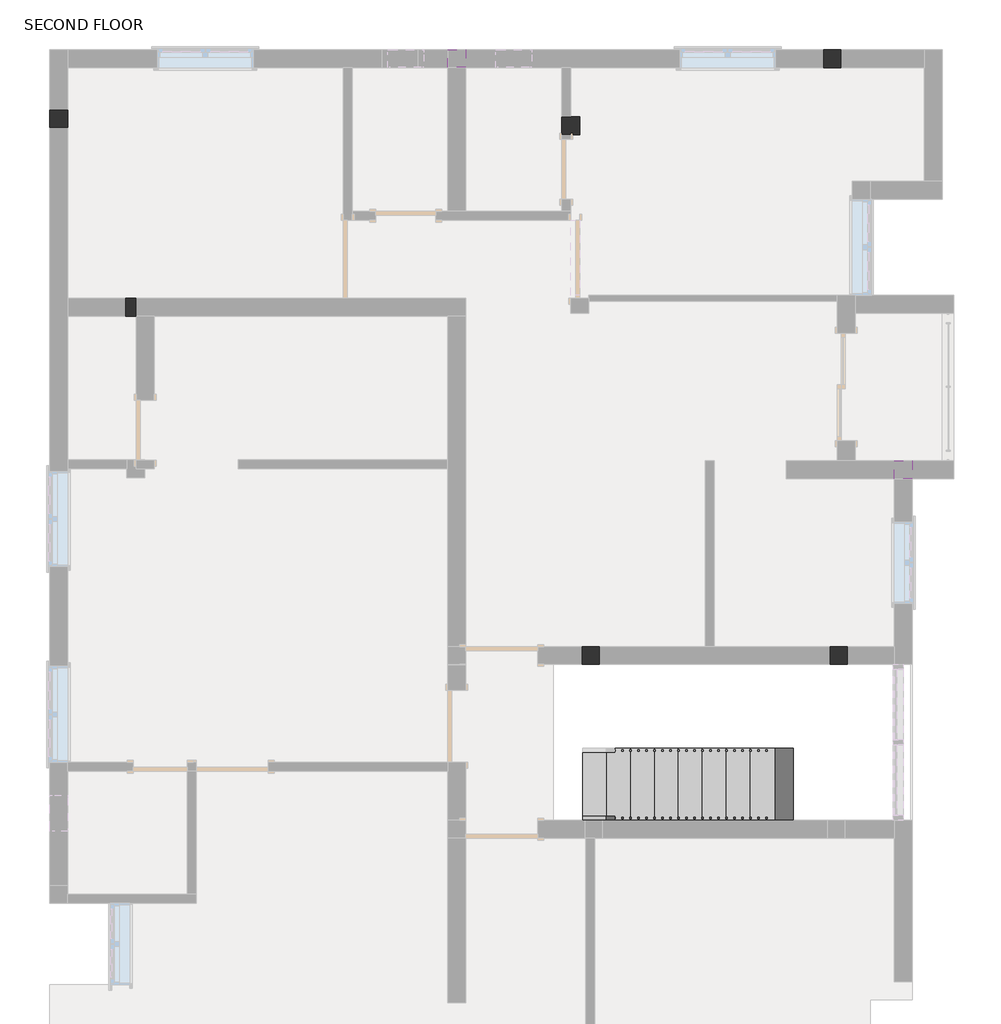
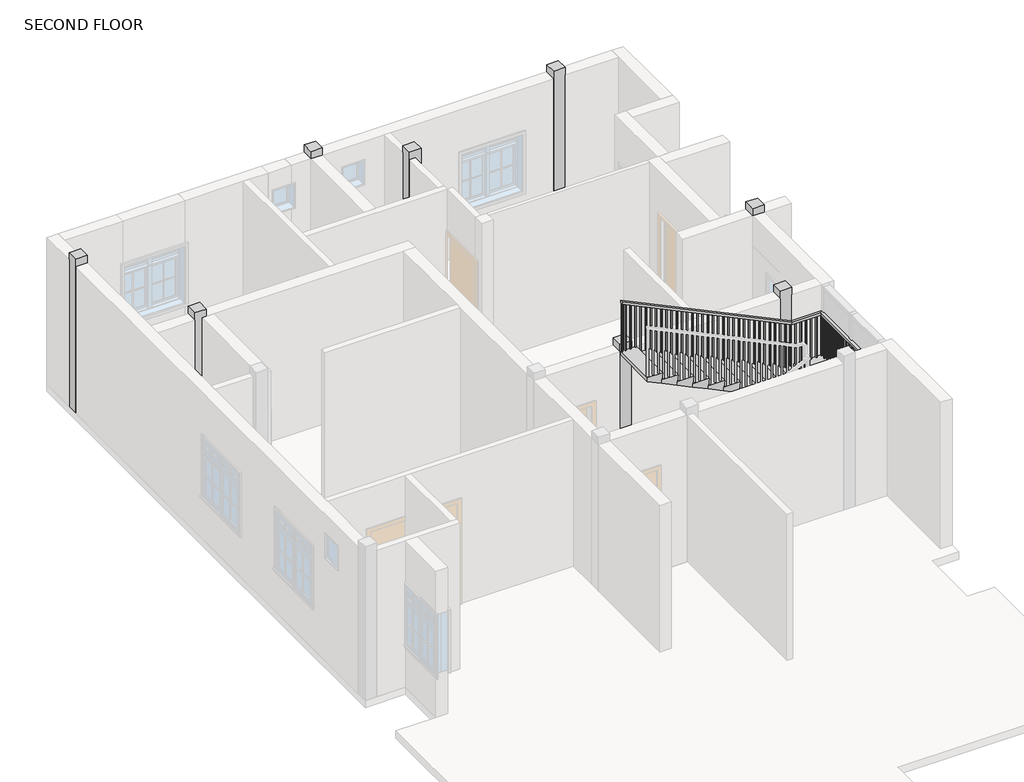
# One storey, part 4 of 6: 8 columns, 1 railing, 1 stair flight.
"""IFC4 building model written with IfcOpenShell, lengths in millimetres."""

from ifc_helpers import new_model, si_unit, frame, origin, place, context, project, spatial, polyline, outline, extrude, faceted_brep, element, save

model = new_model("IFC4")

# Units and contexts
model_context = context("Model", 3, world=origin())
ifc_project = project(units=[si_unit("LENGTHUNIT", "METRE", prefix="MILLI")], contexts=[model_context])

# Site, building, storey
site = spatial("IfcSite", under=ifc_project)
building = spatial("IfcBuilding", under=site)
storey = spatial("IfcBuildingStorey", under=building, Name="SECOND FLOOR", Elevation=6400.8)

# Columns
placement = place(None, origin())
element("IfcColumn", 1, ObjectType="Rectangular Column : 9\"X9\"", at=placement, inside=storey, context=model_context, shape_type="Brep", body=[
    faceted_brep([(-6539.8865981, 8531.2343988, 6400.8), (-6539.8865981, 8302.6343988, 6400.8), (-6768.4865981, 8302.6343988, 6400.8), (-6768.4865981, 8531.2343988, 6400.8), (-6539.8865981, 8531.2343988, 9601.2), (-6539.8865981, 8302.6343988, 9601.2), (-6539.8865981, 8302.6343988, 9448.8), (-6539.8865981, 8531.2343988, 9448.8), (-6768.4865981, 8302.6343988, 9601.2), (-6768.4865981, 8302.6343988, 9448.8), (-6768.4865981, 8531.2343988, 9601.2), (-6768.4865981, 8531.2343988, 9448.8)], [[[0, 1, 2, 3]], [[4, 5, 6, 1, 0, 7]], [[5, 8, 9, 2, 1, 6]], [[8, 10, 11, 3, 2, 9]], [[10, 4, 7, 0, 3, 11]], [[4, 10, 8, 5]]]),
])
element("IfcColumn", 2, ObjectType="Rectangular Column : 9\"X9\"", at=placement, inside=storey, context=model_context, shape_type="Brep", body=[
    faceted_brep([(229.251657, 1705.5787587, 6400.8), (229.251657, 1476.9787587, 6400.8), (0.651657, 1476.9787587, 6400.8), (0.651657, 1705.5787587, 6400.8), (229.251657, 1705.5787587, 9601.2), (229.251657, 1476.9787587, 9601.2), (229.251657, 1476.9787587, 9448.8), (229.251657, 1705.5787587, 9448.8), (0.651657, 1476.9787587, 9601.2), (0.651657, 1476.9787587, 9448.8), (0.651657, 1705.5787587, 9601.2), (0.651657, 1705.5787587, 9448.8)], [[[0, 1, 2, 3]], [[4, 5, 6, 1, 0, 7]], [[5, 8, 9, 2, 1, 6]], [[8, 10, 11, 3, 2, 9]], [[10, 4, 7, 0, 3, 11]], [[4, 10, 8, 5]]]),
])
element("IfcColumn", 3, ObjectType="Rectangular Column : 9\"X9\"", at=placement, inside=storey, context=model_context, shape_type="Brep", body=[
    faceted_brep([(3385.1070369, 1705.5787587, 6400.8), (3385.1070369, 1476.9787587, 6400.8), (3156.5070369, 1476.9787587, 6400.8), (3156.5070369, 1705.5787587, 6400.8), (3385.1070369, 1705.5787587, 9601.2), (3385.1070369, 1476.9787587, 9601.2), (3385.1070369, 1476.9787587, 9448.8), (3385.1070369, 1705.5787587, 9448.8), (3156.5070369, 1476.9787587, 9601.2), (3156.5070369, 1476.9787587, 9448.8), (3156.5070369, 1705.5787587, 9601.2), (3156.5070369, 1705.5787587, 9448.8)], [[[0, 1, 2, 3]], [[4, 5, 6, 1, 0, 7]], [[5, 8, 9, 2, 1, 6]], [[8, 10, 11, 3, 2, 9]], [[10, 4, 7, 0, 3, 11]], [[4, 10, 8, 5]]]),
])
element("IfcColumn", 4, ObjectType="Rectangular Column : 9\"X9\"", at=placement, inside=storey, context=model_context, shape_type="SweptSolid", body=[
    extrude(outline(polyline([(4204.3134019, 4067.7787587), (4204.3134019, 3839.1787587), (3975.7134019, 3839.1787587), (3975.7134019, 4067.7787587), (4204.3134019, 4067.7787587)])), frame((0.0, 0.0, 9448.8), z_axis=(0.0, 0.0, 1.0), x_axis=(1.0, 0.0, 0.0)), (0.0, 0.0, 1.0), 152.4),
])
element("IfcColumn", 5, ObjectType="Rectangular Column : 9\"X9\"", at=placement, inside=storey, context=model_context, shape_type="Brep", body=[
    faceted_brep([(3305.8577655, 9300.1787587, 6400.8), (3305.8577655, 9071.5787587, 6400.8), (3077.2577655, 9071.5787587, 6400.8), (3077.2577655, 9300.1787587, 6400.8), (3305.8577655, 9300.1787587, 9601.2), (3305.8577655, 9071.5787587, 9601.2), (3305.8577655, 9071.5787587, 9448.8), (3305.8577655, 9300.1787587, 9448.8), (3077.2577655, 9071.5787587, 9601.2), (3077.2577655, 9071.5787587, 9448.8), (3077.2577655, 9300.1787587, 9601.2), (3077.2577655, 9300.1787587, 9448.8)], [[[0, 1, 2, 3]], [[4, 5, 6, 1, 0, 7]], [[5, 8, 9, 2, 1, 6]], [[8, 10, 11, 3, 2, 9]], [[10, 4, 7, 0, 3, 11]], [[4, 10, 8, 5]]]),
])
element("IfcColumn", 6, ObjectType="Rectangular Column : 9\"X9\"", at=placement, inside=storey, context=model_context, shape_type="Brep", body=[
    faceted_brep([(-24.7865981, 8443.0921256, 6400.8), (-24.7865981, 8214.4921256, 6400.8), (-139.0865981, 8214.4921256, 6400.8), (-253.3865981, 8214.4921256, 6400.8), (-253.3865981, 8443.0921256, 6400.8), (-139.0865981, 8443.0921256, 6400.8), (-24.7865981, 8443.0921256, 9601.2), (-24.7865981, 8214.4921256, 9601.2), (-253.3865981, 8214.4921256, 9601.2), (-253.3865981, 8214.4921256, 9448.8), (-253.3865981, 8443.0921256, 9601.2), (-253.3865981, 8443.0921256, 9448.8)], [[[0, 1, 2, 3, 4, 5]], [[6, 7, 1, 0]], [[7, 8, 9, 3, 2, 1]], [[8, 10, 11, 4, 3, 9]], [[10, 6, 0, 5, 4, 11]], [[6, 10, 8, 7]]]),
])
element("IfcColumn", 7, ObjectType="Rectangular Column : 9\"X9\"", at=placement, inside=storey, context=model_context, shape_type="Brep", body=[
    faceted_brep([(-5807.056564, 5909.2787587, 6400.8), (-5807.056564, 6137.8787587, 6400.8), (-5663.5865981, 6137.8787587, 6400.8), (-5663.5865981, 5909.2787587, 6400.8), (-5578.456564, 6137.8787587, 9601.2), (-5578.456564, 5909.2787587, 9601.2), (-5578.456564, 5909.2787587, 9448.8), (-5578.456564, 6137.8787587, 9448.8), (-5807.056564, 5909.2787587, 9601.2), (-5807.056564, 5909.2787587, 9448.8), (-5663.5865981, 5909.2787587, 9448.8), (-5807.056564, 6137.8787587, 9601.2), (-5807.056564, 6137.8787587, 9448.8), (-5663.5865981, 6137.8787587, 9448.8)], [[[0, 1, 2, 3]], [[4, 5, 6, 7]], [[5, 8, 9, 0, 3, 10, 6]], [[1, 0, 9, 8, 11, 12]], [[1, 12, 11, 4, 7, 13, 2]], [[5, 4, 11, 8]], [[10, 13, 7, 6]], [[13, 10, 3, 2]]]),
])
element("IfcColumn", 8, ObjectType="Rectangular Column : 9\"X9\"", at=placement, inside=storey, context=model_context, shape_type="SweptSolid", body=[
    extrude(outline(polyline([(-1472.5865981, 9300.1787587), (-1472.5865981, 9071.5787587), (-1701.1865981, 9071.5787587), (-1701.1865981, 9300.1787587), (-1472.5865981, 9300.1787587)])), frame((0.0, 0.0, 9448.8), z_axis=(0.0, 0.0, 1.0), x_axis=(1.0, 0.0, 0.0)), (0.0, 0.0, 1.0), 152.4),
])

# Railing
element("IfcRailing", 9, ObjectType="Handrail - Rectangular", at=placement, inside=storey, context=model_context, shape_type="SolidModel", body=[
    faceted_brep([(13.3134019, -453.4212413, 7460.6727273), (13.3134019, -453.4212413, 7404.3834559), (13.3134019, -504.2212413, 7404.3834559), (13.3134019, -504.2212413, 7460.6727273), (3061.3134019, -453.4212413, 8915.4), (3072.8147322, -453.4212413, 8864.6), (3072.8147322, -504.2212413, 8864.6), (3061.3134019, -504.2212413, 8915.4), (3924.9134019, -453.4212413, 8915.4), (3924.9134019, -453.4212413, 8864.6), (3975.7134019, -504.2212413, 8864.6), (3975.7134019, -504.2212413, 8915.4), (3924.9134019, 1426.1787587, 8915.4), (3924.9134019, 1426.1787587, 8864.6), (3975.7134019, 1476.9787587, 8864.6), (3975.7134019, 1476.9787587, 8915.4), (3366.1134019, 1426.1787587, 8915.4), (3354.6120715, 1426.1787587, 8864.6), (3354.6120715, 1476.9787587, 8864.6), (3366.1134019, 1476.9787587, 8915.4), (13.3134019, 1426.1787587, 10515.6), (13.3134019, 1476.9787587, 10515.6), (13.3134019, 1476.9787587, 10459.3107287), (13.3134019, 1426.1787587, 10459.3107287)], [[[0, 1, 2, 3]], [[1, 0, 4, 5]], [[2, 1, 5, 6]], [[3, 2, 6, 7]], [[0, 3, 7, 4]], [[5, 4, 8, 9]], [[6, 5, 9, 10]], [[7, 6, 10, 11]], [[4, 7, 11, 8]], [[9, 8, 12, 13]], [[10, 9, 13, 14]], [[11, 10, 14, 15]], [[8, 11, 15, 12]], [[13, 12, 16, 17]], [[14, 13, 17, 18]], [[15, 14, 18, 19]], [[12, 15, 19, 16]], [[20, 21, 22, 23]], [[17, 16, 20, 23]], [[18, 17, 23, 22]], [[19, 18, 22, 21]], [[16, 19, 21, 20]]]),
    extrude(outline(polyline([(10418.3965241, 99.0384019), (10427.4885696, 79.9884019), (9455.7272727, 79.9884019), (9455.7272727, 99.0384019), (10418.3965241, 99.0384019)])), frame((0.0, 1442.0537587, 0.0), z_axis=(0.0, 1.0, 0.0), x_axis=(0.0, 0.0, 1.0)), (0.0, 0.0, 1.0), 19.05),
    extrude(outline(polyline([(10369.905615, 200.6384019), (10378.9976605, 181.5884019), (9455.7272727, 181.5884019), (9455.7272727, 200.6384019), (10369.905615, 200.6384019)])), frame((0.0, 1442.0537587, 0.0), z_axis=(0.0, 1.0, 0.0), x_axis=(0.0, 0.0, 1.0)), (0.0, 0.0, 1.0), 19.05),
    extrude(outline(polyline([(10321.4147059, 302.2384019), (10330.5067514, 283.1884019), (9455.7272727, 283.1884019), (9455.7272727, 302.2384019), (10321.4147059, 302.2384019)])), frame((0.0, 1442.0537587, 0.0), z_axis=(0.0, 1.0, 0.0), x_axis=(0.0, 0.0, 1.0)), (0.0, 0.0, 1.0), 19.05),
    extrude(outline(polyline([(10272.9237969, 403.8384019), (10282.0158423, 384.7884019), (9310.2545455, 384.7884019), (9310.2545455, 403.8384019), (10272.9237969, 403.8384019)])), frame((0.0, 1442.0537587, 0.0), z_axis=(0.0, 1.0, 0.0), x_axis=(0.0, 0.0, 1.0)), (0.0, 0.0, 1.0), 19.05),
    extrude(outline(polyline([(10224.4328878, 505.4384019), (10233.5249332, 486.3884019), (9310.2545455, 486.3884019), (9310.2545455, 505.4384019), (10224.4328878, 505.4384019)])), frame((0.0, 1442.0537587, 0.0), z_axis=(0.0, 1.0, 0.0), x_axis=(0.0, 0.0, 1.0)), (0.0, 0.0, 1.0), 19.05),
    extrude(outline(polyline([(10175.9419787, 607.0384019), (10185.0340241, 587.9884019), (9310.2545455, 587.9884019), (9310.2545455, 607.0384019), (10175.9419787, 607.0384019)])), frame((0.0, 1442.0537587, 0.0), z_axis=(0.0, 1.0, 0.0), x_axis=(0.0, 0.0, 1.0)), (0.0, 0.0, 1.0), 19.05),
    extrude(outline(polyline([(10127.4510696, 708.6384019), (10136.543115, 689.5884019), (9164.7818182, 689.5884019), (9164.7818182, 708.6384019), (10127.4510696, 708.6384019)])), frame((0.0, 1442.0537587, 0.0), z_axis=(0.0, 1.0, 0.0), x_axis=(0.0, 0.0, 1.0)), (0.0, 0.0, 1.0), 19.05),
    extrude(outline(polyline([(10078.9601605, 810.2384019), (10088.0522059, 791.1884019), (9164.7818182, 791.1884019), (9164.7818182, 810.2384019), (10078.9601605, 810.2384019)])), frame((0.0, 1442.0537587, 0.0), z_axis=(0.0, 1.0, 0.0), x_axis=(0.0, 0.0, 1.0)), (0.0, 0.0, 1.0), 19.05),
    extrude(outline(polyline([(10030.4692514, 911.8384019), (10039.5612969, 892.7884019), (9164.7818182, 892.7884019), (9164.7818182, 911.8384019), (10030.4692514, 911.8384019)])), frame((0.0, 1442.0537587, 0.0), z_axis=(0.0, 1.0, 0.0), x_axis=(0.0, 0.0, 1.0)), (0.0, 0.0, 1.0), 19.05),
    extrude(outline(polyline([(9981.9783423, 1013.4384019), (9991.0703878, 994.3884019), (9019.3090909, 994.3884019), (9019.3090909, 1013.4384019), (9981.9783423, 1013.4384019)])), frame((0.0, 1442.0537587, 0.0), z_axis=(0.0, 1.0, 0.0), x_axis=(0.0, 0.0, 1.0)), (0.0, 0.0, 1.0), 19.05),
    extrude(outline(polyline([(9933.4874332, 1115.0384019), (9942.5794787, 1095.9884019), (9019.3090909, 1095.9884019), (9019.3090909, 1115.0384019), (9933.4874332, 1115.0384019)])), frame((0.0, 1442.0537587, 0.0), z_axis=(0.0, 1.0, 0.0), x_axis=(0.0, 0.0, 1.0)), (0.0, 0.0, 1.0), 19.05),
    extrude(outline(polyline([(9884.9965241, 1216.6384019), (9894.0885696, 1197.5884019), (9019.3090909, 1197.5884019), (9019.3090909, 1216.6384019), (9884.9965241, 1216.6384019)])), frame((0.0, 1442.0537587, 0.0), z_axis=(0.0, 1.0, 0.0), x_axis=(0.0, 0.0, 1.0)), (0.0, 0.0, 1.0), 19.05),
    extrude(outline(polyline([(9836.505615, 1318.2384019), (9845.5976605, 1299.1884019), (8873.8363636, 1299.1884019), (8873.8363636, 1318.2384019), (9836.505615, 1318.2384019)])), frame((0.0, 1442.0537587, 0.0), z_axis=(0.0, 1.0, 0.0), x_axis=(0.0, 0.0, 1.0)), (0.0, 0.0, 1.0), 19.05),
    extrude(outline(polyline([(9788.0147059, 1419.8384019), (9797.1067514, 1400.7884019), (8873.8363636, 1400.7884019), (8873.8363636, 1419.8384019), (9788.0147059, 1419.8384019)])), frame((0.0, 1442.0537587, 0.0), z_axis=(0.0, 1.0, 0.0), x_axis=(0.0, 0.0, 1.0)), (0.0, 0.0, 1.0), 19.05),
    extrude(outline(polyline([(9739.5237969, 1521.4384019), (9748.6158423, 1502.3884019), (8873.8363636, 1502.3884019), (8873.8363636, 1521.4384019), (9739.5237969, 1521.4384019)])), frame((0.0, 1442.0537587, 0.0), z_axis=(0.0, 1.0, 0.0), x_axis=(0.0, 0.0, 1.0)), (0.0, 0.0, 1.0), 19.05),
    extrude(outline(polyline([(9691.0328878, 1623.0384019), (9700.1249332, 1603.9884019), (8728.3636364, 1603.9884019), (8728.3636364, 1623.0384019), (9691.0328878, 1623.0384019)])), frame((0.0, 1442.0537587, 0.0), z_axis=(0.0, 1.0, 0.0), x_axis=(0.0, 0.0, 1.0)), (0.0, 0.0, 1.0), 19.05),
    extrude(outline(polyline([(9642.5419787, 1724.6384019), (9651.6340241, 1705.5884019), (8728.3636364, 1705.5884019), (8728.3636364, 1724.6384019), (9642.5419787, 1724.6384019)])), frame((0.0, 1442.0537587, 0.0), z_axis=(0.0, 1.0, 0.0), x_axis=(0.0, 0.0, 1.0)), (0.0, 0.0, 1.0), 19.05),
    extrude(outline(polyline([(9594.0510696, 1826.2384019), (9603.143115, 1807.1884019), (8728.3636364, 1807.1884019), (8728.3636364, 1826.2384019), (9594.0510696, 1826.2384019)])), frame((0.0, 1442.0537587, 0.0), z_axis=(0.0, 1.0, 0.0), x_axis=(0.0, 0.0, 1.0)), (0.0, 0.0, 1.0), 19.05),
    extrude(outline(polyline([(9545.5601605, 1927.8384019), (9554.6522059, 1908.7884019), (8582.8909091, 1908.7884019), (8582.8909091, 1927.8384019), (9545.5601605, 1927.8384019)])), frame((0.0, 1442.0537587, 0.0), z_axis=(0.0, 1.0, 0.0), x_axis=(0.0, 0.0, 1.0)), (0.0, 0.0, 1.0), 19.05),
    extrude(outline(polyline([(9497.0692514, 2029.4384019), (9506.1612969, 2010.3884019), (8582.8909091, 2010.3884019), (8582.8909091, 2029.4384019), (9497.0692514, 2029.4384019)])), frame((0.0, 1442.0537587, 0.0), z_axis=(0.0, 1.0, 0.0), x_axis=(0.0, 0.0, 1.0)), (0.0, 0.0, 1.0), 19.05),
    extrude(outline(polyline([(9448.5783423, 2131.0384019), (9457.6703878, 2111.9884019), (8582.8909091, 2111.9884019), (8582.8909091, 2131.0384019), (9448.5783423, 2131.0384019)])), frame((0.0, 1442.0537587, 0.0), z_axis=(0.0, 1.0, 0.0), x_axis=(0.0, 0.0, 1.0)), (0.0, 0.0, 1.0), 19.05),
    extrude(outline(polyline([(9400.0874332, 2232.6384019), (9409.1794787, 2213.5884019), (8437.4181818, 2213.5884019), (8437.4181818, 2232.6384019), (9400.0874332, 2232.6384019)])), frame((0.0, 1442.0537587, 0.0), z_axis=(0.0, 1.0, 0.0), x_axis=(0.0, 0.0, 1.0)), (0.0, 0.0, 1.0), 19.05),
    extrude(outline(polyline([(9351.5965241, 2334.2384019), (9360.6885696, 2315.1884019), (8437.4181818, 2315.1884019), (8437.4181818, 2334.2384019), (9351.5965241, 2334.2384019)])), frame((0.0, 1442.0537587, 0.0), z_axis=(0.0, 1.0, 0.0), x_axis=(0.0, 0.0, 1.0)), (0.0, 0.0, 1.0), 19.05),
    extrude(outline(polyline([(9303.105615, 2435.8384019), (9312.1976605, 2416.7884019), (8437.4181818, 2416.7884019), (8437.4181818, 2435.8384019), (9303.105615, 2435.8384019)])), frame((0.0, 1442.0537587, 0.0), z_axis=(0.0, 1.0, 0.0), x_axis=(0.0, 0.0, 1.0)), (0.0, 0.0, 1.0), 19.05),
    extrude(outline(polyline([(9254.6147059, 2537.4384019), (9263.7067514, 2518.3884019), (8291.9454545, 2518.3884019), (8291.9454545, 2537.4384019), (9254.6147059, 2537.4384019)])), frame((0.0, 1442.0537587, 0.0), z_axis=(0.0, 1.0, 0.0), x_axis=(0.0, 0.0, 1.0)), (0.0, 0.0, 1.0), 19.05),
    extrude(outline(polyline([(9206.1237969, 2639.0384019), (9215.2158423, 2619.9884019), (8291.9454545, 2619.9884019), (8291.9454545, 2639.0384019), (9206.1237969, 2639.0384019)])), frame((0.0, 1442.0537587, 0.0), z_axis=(0.0, 1.0, 0.0), x_axis=(0.0, 0.0, 1.0)), (0.0, 0.0, 1.0), 19.05),
    extrude(outline(polyline([(9157.6328878, 2740.6384019), (9166.7249332, 2721.5884019), (8291.9454545, 2721.5884019), (8291.9454545, 2740.6384019), (9157.6328878, 2740.6384019)])), frame((0.0, 1442.0537587, 0.0), z_axis=(0.0, 1.0, 0.0), x_axis=(0.0, 0.0, 1.0)), (0.0, 0.0, 1.0), 19.05),
    extrude(outline(polyline([(9109.1419787, 2842.2384019), (9118.2340241, 2823.1884019), (8146.4727273, 2823.1884019), (8146.4727273, 2842.2384019), (9109.1419787, 2842.2384019)])), frame((0.0, 1442.0537587, 0.0), z_axis=(0.0, 1.0, 0.0), x_axis=(0.0, 0.0, 1.0)), (0.0, 0.0, 1.0), 19.05),
    extrude(outline(polyline([(9060.6510696, 2943.8384019), (9069.743115, 2924.7884019), (8146.4727273, 2924.7884019), (8146.4727273, 2943.8384019), (9060.6510696, 2943.8384019)])), frame((0.0, 1442.0537587, 0.0), z_axis=(0.0, 1.0, 0.0), x_axis=(0.0, 0.0, 1.0)), (0.0, 0.0, 1.0), 19.05),
    extrude(outline(polyline([(9012.1601605, 3045.4384019), (9021.2522059, 3026.3884019), (8146.4727273, 3026.3884019), (8146.4727273, 3045.4384019), (9012.1601605, 3045.4384019)])), frame((0.0, 1442.0537587, 0.0), z_axis=(0.0, 1.0, 0.0), x_axis=(0.0, 0.0, 1.0)), (0.0, 0.0, 1.0), 19.05),
    extrude(outline(polyline([(8963.6692514, 3147.0384019), (8972.7612969, 3127.9884019), (8001.0, 3127.9884019), (8001.0, 3147.0384019), (8963.6692514, 3147.0384019)])), frame((0.0, 1442.0537587, 0.0), z_axis=(0.0, 1.0, 0.0), x_axis=(0.0, 0.0, 1.0)), (0.0, 0.0, 1.0), 19.05),
    extrude(outline(polyline([(8915.1783423, 3248.6384019), (8924.2703878, 3229.5884019), (8001.0, 3229.5884019), (8001.0, 3248.6384019), (8915.1783423, 3248.6384019)])), frame((0.0, 1442.0537587, 0.0), z_axis=(0.0, 1.0, 0.0), x_axis=(0.0, 0.0, 1.0)), (0.0, 0.0, 1.0), 19.05),
    extrude(outline(polyline([(8866.6874332, 3350.2384019), (8875.7794787, 3331.1884019), (8001.0, 3331.1884019), (8001.0, 3350.2384019), (8866.6874332, 3350.2384019)])), frame((0.0, 1442.0537587, 0.0), z_axis=(0.0, 1.0, 0.0), x_axis=(0.0, 0.0, 1.0)), (0.0, 0.0, 1.0), 19.05),
    extrude(outline(polyline([(3451.8384019, 1461.1037587), (3451.8384019, 1442.0537587), (3432.7884019, 1442.0537587), (3432.7884019, 1461.1037587), (3451.8384019, 1461.1037587)])), frame((0.0, 0.0, 8001.0), z_axis=(0.0, 0.0, 1.0), x_axis=(1.0, 0.0, 0.0)), (0.0, 0.0, 1.0), 863.6),
    extrude(outline(polyline([(3553.4384019, 1461.1037587), (3553.4384019, 1442.0537587), (3534.3884019, 1442.0537587), (3534.3884019, 1461.1037587), (3553.4384019, 1461.1037587)])), frame((0.0, 0.0, 8001.0), z_axis=(0.0, 0.0, 1.0), x_axis=(1.0, 0.0, 0.0)), (0.0, 0.0, 1.0), 863.6),
    extrude(outline(polyline([(3655.0384019, 1461.1037587), (3655.0384019, 1442.0537587), (3635.9884019, 1442.0537587), (3635.9884019, 1461.1037587), (3655.0384019, 1461.1037587)])), frame((0.0, 0.0, 8001.0), z_axis=(0.0, 0.0, 1.0), x_axis=(1.0, 0.0, 0.0)), (0.0, 0.0, 1.0), 863.6),
    extrude(outline(polyline([(3756.6384019, 1461.1037587), (3756.6384019, 1442.0537587), (3737.5884019, 1442.0537587), (3737.5884019, 1461.1037587), (3756.6384019, 1461.1037587)])), frame((0.0, 0.0, 8001.0), z_axis=(0.0, 0.0, 1.0), x_axis=(1.0, 0.0, 0.0)), (0.0, 0.0, 1.0), 863.6),
    extrude(outline(polyline([(3858.2384019, 1461.1037587), (3858.2384019, 1442.0537587), (3839.1884019, 1442.0537587), (3839.1884019, 1461.1037587), (3858.2384019, 1461.1037587)])), frame((0.0, 0.0, 8001.0), z_axis=(0.0, 0.0, 1.0), x_axis=(1.0, 0.0, 0.0)), (0.0, 0.0, 1.0), 863.6),
    extrude(outline(polyline([(3959.8384019, 1340.4537587), (3940.7884019, 1340.4537587), (3940.7884019, 1359.5037587), (3959.8384019, 1359.5037587), (3959.8384019, 1340.4537587)])), frame((0.0, 0.0, 8001.0), z_axis=(0.0, 0.0, 1.0), x_axis=(1.0, 0.0, 0.0)), (0.0, 0.0, 1.0), 863.6),
    extrude(outline(polyline([(3959.8384019, 1238.8537587), (3940.7884019, 1238.8537587), (3940.7884019, 1257.9037587), (3959.8384019, 1257.9037587), (3959.8384019, 1238.8537587)])), frame((0.0, 0.0, 8001.0), z_axis=(0.0, 0.0, 1.0), x_axis=(1.0, 0.0, 0.0)), (0.0, 0.0, 1.0), 863.6),
    extrude(outline(polyline([(3959.8384019, 1137.2537587), (3940.7884019, 1137.2537587), (3940.7884019, 1156.3037587), (3959.8384019, 1156.3037587), (3959.8384019, 1137.2537587)])), frame((0.0, 0.0, 8001.0), z_axis=(0.0, 0.0, 1.0), x_axis=(1.0, 0.0, 0.0)), (0.0, 0.0, 1.0), 863.6),
    extrude(outline(polyline([(3959.8384019, 1035.6537587), (3940.7884019, 1035.6537587), (3940.7884019, 1054.7037587), (3959.8384019, 1054.7037587), (3959.8384019, 1035.6537587)])), frame((0.0, 0.0, 8001.0), z_axis=(0.0, 0.0, 1.0), x_axis=(1.0, 0.0, 0.0)), (0.0, 0.0, 1.0), 863.6),
    extrude(outline(polyline([(3959.8384019, 934.0537587), (3940.7884019, 934.0537587), (3940.7884019, 953.1037587), (3959.8384019, 953.1037587), (3959.8384019, 934.0537587)])), frame((0.0, 0.0, 8001.0), z_axis=(0.0, 0.0, 1.0), x_axis=(1.0, 0.0, 0.0)), (0.0, 0.0, 1.0), 863.6),
    extrude(outline(polyline([(3959.8384019, 832.4537587), (3940.7884019, 832.4537587), (3940.7884019, 851.5037587), (3959.8384019, 851.5037587), (3959.8384019, 832.4537587)])), frame((0.0, 0.0, 8001.0), z_axis=(0.0, 0.0, 1.0), x_axis=(1.0, 0.0, 0.0)), (0.0, 0.0, 1.0), 863.6),
    extrude(outline(polyline([(3959.8384019, 730.8537587), (3940.7884019, 730.8537587), (3940.7884019, 749.9037587), (3959.8384019, 749.9037587), (3959.8384019, 730.8537587)])), frame((0.0, 0.0, 8001.0), z_axis=(0.0, 0.0, 1.0), x_axis=(1.0, 0.0, 0.0)), (0.0, 0.0, 1.0), 863.6),
    extrude(outline(polyline([(3959.8384019, 629.2537587), (3940.7884019, 629.2537587), (3940.7884019, 648.3037587), (3959.8384019, 648.3037587), (3959.8384019, 629.2537587)])), frame((0.0, 0.0, 8001.0), z_axis=(0.0, 0.0, 1.0), x_axis=(1.0, 0.0, 0.0)), (0.0, 0.0, 1.0), 863.6),
    extrude(outline(polyline([(3959.8384019, 527.6537587), (3940.7884019, 527.6537587), (3940.7884019, 546.7037587), (3959.8384019, 546.7037587), (3959.8384019, 527.6537587)])), frame((0.0, 0.0, 8001.0), z_axis=(0.0, 0.0, 1.0), x_axis=(1.0, 0.0, 0.0)), (0.0, 0.0, 1.0), 863.6),
    extrude(outline(polyline([(3959.8384019, 426.0537587), (3940.7884019, 426.0537587), (3940.7884019, 445.1037587), (3959.8384019, 445.1037587), (3959.8384019, 426.0537587)])), frame((0.0, 0.0, 8001.0), z_axis=(0.0, 0.0, 1.0), x_axis=(1.0, 0.0, 0.0)), (0.0, 0.0, 1.0), 863.6),
    extrude(outline(polyline([(3959.8384019, 324.4537587), (3940.7884019, 324.4537587), (3940.7884019, 343.5037587), (3959.8384019, 343.5037587), (3959.8384019, 324.4537587)])), frame((0.0, 0.0, 8001.0), z_axis=(0.0, 0.0, 1.0), x_axis=(1.0, 0.0, 0.0)), (0.0, 0.0, 1.0), 863.6),
    extrude(outline(polyline([(3959.8384019, 222.8537587), (3940.7884019, 222.8537587), (3940.7884019, 241.9037587), (3959.8384019, 241.9037587), (3959.8384019, 222.8537587)])), frame((0.0, 0.0, 8001.0), z_axis=(0.0, 0.0, 1.0), x_axis=(1.0, 0.0, 0.0)), (0.0, 0.0, 1.0), 863.6),
    extrude(outline(polyline([(3959.8384019, 121.2537587), (3940.7884019, 121.2537587), (3940.7884019, 140.3037587), (3959.8384019, 140.3037587), (3959.8384019, 121.2537587)])), frame((0.0, 0.0, 8001.0), z_axis=(0.0, 0.0, 1.0), x_axis=(1.0, 0.0, 0.0)), (0.0, 0.0, 1.0), 863.6),
    extrude(outline(polyline([(3959.8384019, 19.6537587), (3940.7884019, 19.6537587), (3940.7884019, 38.7037587), (3959.8384019, 38.7037587), (3959.8384019, 19.6537587)])), frame((0.0, 0.0, 8001.0), z_axis=(0.0, 0.0, 1.0), x_axis=(1.0, 0.0, 0.0)), (0.0, 0.0, 1.0), 863.6),
    extrude(outline(polyline([(3959.8384019, -81.9462413), (3940.7884019, -81.9462413), (3940.7884019, -62.8962413), (3959.8384019, -62.8962413), (3959.8384019, -81.9462413)])), frame((0.0, 0.0, 8001.0), z_axis=(0.0, 0.0, 1.0), x_axis=(1.0, 0.0, 0.0)), (0.0, 0.0, 1.0), 863.6),
    extrude(outline(polyline([(3959.8384019, -183.5462413), (3940.7884019, -183.5462413), (3940.7884019, -164.4962413), (3959.8384019, -164.4962413), (3959.8384019, -183.5462413)])), frame((0.0, 0.0, 8001.0), z_axis=(0.0, 0.0, 1.0), x_axis=(1.0, 0.0, 0.0)), (0.0, 0.0, 1.0), 863.6),
    extrude(outline(polyline([(3959.8384019, -285.1462413), (3940.7884019, -285.1462413), (3940.7884019, -266.0962413), (3959.8384019, -266.0962413), (3959.8384019, -285.1462413)])), frame((0.0, 0.0, 8001.0), z_axis=(0.0, 0.0, 1.0), x_axis=(1.0, 0.0, 0.0)), (0.0, 0.0, 1.0), 863.6),
    extrude(outline(polyline([(3959.8384019, -386.7462413), (3940.7884019, -386.7462413), (3940.7884019, -367.6962413), (3959.8384019, -367.6962413), (3959.8384019, -386.7462413)])), frame((0.0, 0.0, 8001.0), z_axis=(0.0, 0.0, 1.0), x_axis=(1.0, 0.0, 0.0)), (0.0, 0.0, 1.0), 863.6),
    extrude(outline(polyline([(3864.5884019, -488.3462413), (3864.5884019, -469.2962413), (3883.6384019, -469.2962413), (3883.6384019, -488.3462413), (3864.5884019, -488.3462413)])), frame((0.0, 0.0, 8001.0), z_axis=(0.0, 0.0, 1.0), x_axis=(1.0, 0.0, 0.0)), (0.0, 0.0, 1.0), 863.6),
    extrude(outline(polyline([(3762.9884019, -488.3462413), (3762.9884019, -469.2962413), (3782.0384019, -469.2962413), (3782.0384019, -488.3462413), (3762.9884019, -488.3462413)])), frame((0.0, 0.0, 8001.0), z_axis=(0.0, 0.0, 1.0), x_axis=(1.0, 0.0, 0.0)), (0.0, 0.0, 1.0), 863.6),
    extrude(outline(polyline([(3661.3884019, -488.3462413), (3661.3884019, -469.2962413), (3680.4384019, -469.2962413), (3680.4384019, -488.3462413), (3661.3884019, -488.3462413)])), frame((0.0, 0.0, 8001.0), z_axis=(0.0, 0.0, 1.0), x_axis=(1.0, 0.0, 0.0)), (0.0, 0.0, 1.0), 863.6),
    extrude(outline(polyline([(3559.7884019, -488.3462413), (3559.7884019, -469.2962413), (3578.8384019, -469.2962413), (3578.8384019, -488.3462413), (3559.7884019, -488.3462413)])), frame((0.0, 0.0, 8001.0), z_axis=(0.0, 0.0, 1.0), x_axis=(1.0, 0.0, 0.0)), (0.0, 0.0, 1.0), 863.6),
    extrude(outline(polyline([(3458.1884019, -488.3462413), (3458.1884019, -469.2962413), (3477.2384019, -469.2962413), (3477.2384019, -488.3462413), (3458.1884019, -488.3462413)])), frame((0.0, 0.0, 8001.0), z_axis=(0.0, 0.0, 1.0), x_axis=(1.0, 0.0, 0.0)), (0.0, 0.0, 1.0), 863.6),
    extrude(outline(polyline([(3356.5884019, -488.3462413), (3356.5884019, -469.2962413), (3375.6384019, -469.2962413), (3375.6384019, -488.3462413), (3356.5884019, -488.3462413)])), frame((0.0, 0.0, 8001.0), z_axis=(0.0, 0.0, 1.0), x_axis=(1.0, 0.0, 0.0)), (0.0, 0.0, 1.0), 863.6),
    extrude(outline(polyline([(3254.9884019, -488.3462413), (3254.9884019, -469.2962413), (3274.0384019, -469.2962413), (3274.0384019, -488.3462413), (3254.9884019, -488.3462413)])), frame((0.0, 0.0, 8001.0), z_axis=(0.0, 0.0, 1.0), x_axis=(1.0, 0.0, 0.0)), (0.0, 0.0, 1.0), 863.6),
    extrude(outline(polyline([(3153.3884019, -488.3462413), (3153.3884019, -469.2962413), (3172.4384019, -469.2962413), (3172.4384019, -488.3462413), (3153.3884019, -488.3462413)])), frame((0.0, 0.0, 8001.0), z_axis=(0.0, 0.0, 1.0), x_axis=(1.0, 0.0, 0.0)), (0.0, 0.0, 1.0), 863.6),
    extrude(outline(polyline([(8863.6567514, 3070.8384019), (8854.5647059, 3051.7884019), (8001.0, 3051.7884019), (8001.0, 3070.8384019), (8863.6567514, 3070.8384019)])), frame((0.0, -488.3462413, 0.0), z_axis=(0.0, 1.0, 0.0), x_axis=(0.0, 0.0, 1.0)), (0.0, 0.0, 1.0), 19.05),
    extrude(outline(polyline([(8815.1658423, 2969.2384019), (8806.0737969, 2950.1884019), (7855.5272727, 2950.1884019), (7855.5272727, 2969.2384019), (8815.1658423, 2969.2384019)])), frame((0.0, -488.3462413, 0.0), z_axis=(0.0, 1.0, 0.0), x_axis=(0.0, 0.0, 1.0)), (0.0, 0.0, 1.0), 19.05),
    extrude(outline(polyline([(8766.6749332, 2867.6384019), (8757.5828878, 2848.5884019), (7855.5272727, 2848.5884019), (7855.5272727, 2867.6384019), (8766.6749332, 2867.6384019)])), frame((0.0, -488.3462413, 0.0), z_axis=(0.0, 1.0, 0.0), x_axis=(0.0, 0.0, 1.0)), (0.0, 0.0, 1.0), 19.05),
    extrude(outline(polyline([(8718.1840241, 2766.0384019), (8709.0919787, 2746.9884019), (7855.5272727, 2746.9884019), (7855.5272727, 2766.0384019), (8718.1840241, 2766.0384019)])), frame((0.0, -488.3462413, 0.0), z_axis=(0.0, 1.0, 0.0), x_axis=(0.0, 0.0, 1.0)), (0.0, 0.0, 1.0), 19.05),
    extrude(outline(polyline([(8669.693115, 2664.4384019), (8660.6010696, 2645.3884019), (7710.0545455, 2645.3884019), (7710.0545455, 2664.4384019), (8669.693115, 2664.4384019)])), frame((0.0, -488.3462413, 0.0), z_axis=(0.0, 1.0, 0.0), x_axis=(0.0, 0.0, 1.0)), (0.0, 0.0, 1.0), 19.05),
    extrude(outline(polyline([(8621.2022059, 2562.8384019), (8612.1101605, 2543.7884019), (7710.0545455, 2543.7884019), (7710.0545455, 2562.8384019), (8621.2022059, 2562.8384019)])), frame((0.0, -488.3462413, 0.0), z_axis=(0.0, 1.0, 0.0), x_axis=(0.0, 0.0, 1.0)), (0.0, 0.0, 1.0), 19.05),
    extrude(outline(polyline([(8572.7112969, 2461.2384019), (8563.6192514, 2442.1884019), (7710.0545455, 2442.1884019), (7710.0545455, 2461.2384019), (8572.7112969, 2461.2384019)])), frame((0.0, -488.3462413, 0.0), z_axis=(0.0, 1.0, 0.0), x_axis=(0.0, 0.0, 1.0)), (0.0, 0.0, 1.0), 19.05),
    extrude(outline(polyline([(8524.2203878, 2359.6384019), (8515.1283423, 2340.5884019), (7564.5818182, 2340.5884019), (7564.5818182, 2359.6384019), (8524.2203878, 2359.6384019)])), frame((0.0, -488.3462413, 0.0), z_axis=(0.0, 1.0, 0.0), x_axis=(0.0, 0.0, 1.0)), (0.0, 0.0, 1.0), 19.05),
    extrude(outline(polyline([(8475.7294787, 2258.0384019), (8466.6374332, 2238.9884019), (7564.5818182, 2238.9884019), (7564.5818182, 2258.0384019), (8475.7294787, 2258.0384019)])), frame((0.0, -488.3462413, 0.0), z_axis=(0.0, 1.0, 0.0), x_axis=(0.0, 0.0, 1.0)), (0.0, 0.0, 1.0), 19.05),
    extrude(outline(polyline([(8427.2385696, 2156.4384019), (8418.1465241, 2137.3884019), (7564.5818182, 2137.3884019), (7564.5818182, 2156.4384019), (8427.2385696, 2156.4384019)])), frame((0.0, -488.3462413, 0.0), z_axis=(0.0, 1.0, 0.0), x_axis=(0.0, 0.0, 1.0)), (0.0, 0.0, 1.0), 19.05),
    extrude(outline(polyline([(8378.7476605, 2054.8384019), (8369.655615, 2035.7884019), (7419.1090909, 2035.7884019), (7419.1090909, 2054.8384019), (8378.7476605, 2054.8384019)])), frame((0.0, -488.3462413, 0.0), z_axis=(0.0, 1.0, 0.0), x_axis=(0.0, 0.0, 1.0)), (0.0, 0.0, 1.0), 19.05),
    extrude(outline(polyline([(8330.2567514, 1953.2384019), (8321.1647059, 1934.1884019), (7419.1090909, 1934.1884019), (7419.1090909, 1953.2384019), (8330.2567514, 1953.2384019)])), frame((0.0, -488.3462413, 0.0), z_axis=(0.0, 1.0, 0.0), x_axis=(0.0, 0.0, 1.0)), (0.0, 0.0, 1.0), 19.05),
    extrude(outline(polyline([(8281.7658423, 1851.6384019), (8272.6737969, 1832.5884019), (7419.1090909, 1832.5884019), (7419.1090909, 1851.6384019), (8281.7658423, 1851.6384019)])), frame((0.0, -488.3462413, 0.0), z_axis=(0.0, 1.0, 0.0), x_axis=(0.0, 0.0, 1.0)), (0.0, 0.0, 1.0), 19.05),
    extrude(outline(polyline([(8233.2749332, 1750.0384019), (8224.1828878, 1730.9884019), (7273.6363636, 1730.9884019), (7273.6363636, 1750.0384019), (8233.2749332, 1750.0384019)])), frame((0.0, -488.3462413, 0.0), z_axis=(0.0, 1.0, 0.0), x_axis=(0.0, 0.0, 1.0)), (0.0, 0.0, 1.0), 19.05),
    extrude(outline(polyline([(8184.7840241, 1648.4384019), (8175.6919787, 1629.3884019), (7273.6363636, 1629.3884019), (7273.6363636, 1648.4384019), (8184.7840241, 1648.4384019)])), frame((0.0, -488.3462413, 0.0), z_axis=(0.0, 1.0, 0.0), x_axis=(0.0, 0.0, 1.0)), (0.0, 0.0, 1.0), 19.05),
    extrude(outline(polyline([(8136.293115, 1546.8384019), (8127.2010696, 1527.7884019), (7273.6363636, 1527.7884019), (7273.6363636, 1546.8384019), (8136.293115, 1546.8384019)])), frame((0.0, -488.3462413, 0.0), z_axis=(0.0, 1.0, 0.0), x_axis=(0.0, 0.0, 1.0)), (0.0, 0.0, 1.0), 19.05),
    extrude(outline(polyline([(8087.8022059, 1445.2384019), (8078.7101605, 1426.1884019), (7128.1636364, 1426.1884019), (7128.1636364, 1445.2384019), (8087.8022059, 1445.2384019)])), frame((0.0, -488.3462413, 0.0), z_axis=(0.0, 1.0, 0.0), x_axis=(0.0, 0.0, 1.0)), (0.0, 0.0, 1.0), 19.05),
    extrude(outline(polyline([(8039.3112969, 1343.6384019), (8030.2192514, 1324.5884019), (7128.1636364, 1324.5884019), (7128.1636364, 1343.6384019), (8039.3112969, 1343.6384019)])), frame((0.0, -488.3462413, 0.0), z_axis=(0.0, 1.0, 0.0), x_axis=(0.0, 0.0, 1.0)), (0.0, 0.0, 1.0), 19.05),
    extrude(outline(polyline([(7990.8203878, 1242.0384019), (7981.7283423, 1222.9884019), (7128.1636364, 1222.9884019), (7128.1636364, 1242.0384019), (7990.8203878, 1242.0384019)])), frame((0.0, -488.3462413, 0.0), z_axis=(0.0, 1.0, 0.0), x_axis=(0.0, 0.0, 1.0)), (0.0, 0.0, 1.0), 19.05),
    extrude(outline(polyline([(7942.3294787, 1140.4384019), (7933.2374332, 1121.3884019), (6982.6909091, 1121.3884019), (6982.6909091, 1140.4384019), (7942.3294787, 1140.4384019)])), frame((0.0, -488.3462413, 0.0), z_axis=(0.0, 1.0, 0.0), x_axis=(0.0, 0.0, 1.0)), (0.0, 0.0, 1.0), 19.05),
    extrude(outline(polyline([(7893.8385696, 1038.8384019), (7884.7465241, 1019.7884019), (6982.6909091, 1019.7884019), (6982.6909091, 1038.8384019), (7893.8385696, 1038.8384019)])), frame((0.0, -488.3462413, 0.0), z_axis=(0.0, 1.0, 0.0), x_axis=(0.0, 0.0, 1.0)), (0.0, 0.0, 1.0), 19.05),
    extrude(outline(polyline([(7845.3476605, 937.2384019), (7836.255615, 918.1884019), (6982.6909091, 918.1884019), (6982.6909091, 937.2384019), (7845.3476605, 937.2384019)])), frame((0.0, -488.3462413, 0.0), z_axis=(0.0, 1.0, 0.0), x_axis=(0.0, 0.0, 1.0)), (0.0, 0.0, 1.0), 19.05),
    extrude(outline(polyline([(7796.8567514, 835.6384019), (7787.7647059, 816.5884019), (6837.2181818, 816.5884019), (6837.2181818, 835.6384019), (7796.8567514, 835.6384019)])), frame((0.0, -488.3462413, 0.0), z_axis=(0.0, 1.0, 0.0), x_axis=(0.0, 0.0, 1.0)), (0.0, 0.0, 1.0), 19.05),
    extrude(outline(polyline([(7748.3658423, 734.0384019), (7739.2737969, 714.9884019), (6837.2181818, 714.9884019), (6837.2181818, 734.0384019), (7748.3658423, 734.0384019)])), frame((0.0, -488.3462413, 0.0), z_axis=(0.0, 1.0, 0.0), x_axis=(0.0, 0.0, 1.0)), (0.0, 0.0, 1.0), 19.05),
    extrude(outline(polyline([(7699.8749332, 632.4384019), (7690.7828878, 613.3884019), (6837.2181818, 613.3884019), (6837.2181818, 632.4384019), (7699.8749332, 632.4384019)])), frame((0.0, -488.3462413, 0.0), z_axis=(0.0, 1.0, 0.0), x_axis=(0.0, 0.0, 1.0)), (0.0, 0.0, 1.0), 19.05),
    extrude(outline(polyline([(7651.3840241, 530.8384019), (7642.2919787, 511.7884019), (6691.7454545, 511.7884019), (6691.7454545, 530.8384019), (7651.3840241, 530.8384019)])), frame((0.0, -488.3462413, 0.0), z_axis=(0.0, 1.0, 0.0), x_axis=(0.0, 0.0, 1.0)), (0.0, 0.0, 1.0), 19.05),
    extrude(outline(polyline([(7602.893115, 429.2384019), (7593.8010696, 410.1884019), (6691.7454545, 410.1884019), (6691.7454545, 429.2384019), (7602.893115, 429.2384019)])), frame((0.0, -488.3462413, 0.0), z_axis=(0.0, 1.0, 0.0), x_axis=(0.0, 0.0, 1.0)), (0.0, 0.0, 1.0), 19.05),
    extrude(outline(polyline([(7554.4022059, 327.6384019), (7545.3101605, 308.5884019), (6691.7454545, 308.5884019), (6691.7454545, 327.6384019), (7554.4022059, 327.6384019)])), frame((0.0, -488.3462413, 0.0), z_axis=(0.0, 1.0, 0.0), x_axis=(0.0, 0.0, 1.0)), (0.0, 0.0, 1.0), 19.05),
    extrude(outline(polyline([(7505.9112969, 226.0384019), (7496.8192514, 206.9884019), (6546.2727273, 206.9884019), (6546.2727273, 226.0384019), (7505.9112969, 226.0384019)])), frame((0.0, -488.3462413, 0.0), z_axis=(0.0, 1.0, 0.0), x_axis=(0.0, 0.0, 1.0)), (0.0, 0.0, 1.0), 19.05),
    extrude(outline(polyline([(7457.4203878, 124.4384019), (7448.3283423, 105.3884019), (6546.2727273, 105.3884019), (6546.2727273, 124.4384019), (7457.4203878, 124.4384019)])), frame((0.0, -488.3462413, 0.0), z_axis=(0.0, 1.0, 0.0), x_axis=(0.0, 0.0, 1.0)), (0.0, 0.0, 1.0), 19.05),
    extrude(outline(polyline([(3959.8384019, 1442.0537587), (3940.7884019, 1442.0537587), (3940.7884019, 1461.1037587), (3959.8384019, 1461.1037587), (3959.8384019, 1442.0537587)])), frame((0.0, 0.0, 8001.0), z_axis=(0.0, 0.0, 1.0), x_axis=(1.0, 0.0, 0.0)), (0.0, 0.0, 1.0), 863.6),
    extrude(outline(polyline([(3940.7884019, -488.3462413), (3940.7884019, -469.2962413), (3959.8384019, -469.2962413), (3959.8384019, -488.3462413), (3940.7884019, -488.3462413)])), frame((0.0, 0.0, 8001.0), z_axis=(0.0, 0.0, 1.0), x_axis=(1.0, 0.0, 0.0)), (0.0, 0.0, 1.0), 863.6),
    extrude(outline(polyline([(10450.2186832, 32.3634019), (10459.3107287, 13.3134019), (9455.7272727, 13.3134019), (9455.7272727, 32.3634019), (10450.2186832, 32.3634019)])), frame((0.0, 1442.0537587, 0.0), z_axis=(0.0, 1.0, 0.0), x_axis=(0.0, 0.0, 1.0)), (0.0, 0.0, 1.0), 19.05),
    extrude(outline(polyline([(7413.4755014, 32.3634019), (7404.3834559, 13.3134019), (6546.2727273, 13.3134019), (6546.2727273, 32.3634019), (7413.4755014, 32.3634019)])), frame((0.0, -488.3462413, 0.0), z_axis=(0.0, 1.0, 0.0), x_axis=(0.0, 0.0, 1.0)), (0.0, 0.0, 1.0), 19.05),
])

# Stair flight
element("IfcStairFlight", 10, ObjectType="3/4\" Nosing", at=placement, inside=storey, context=model_context, shape_type="Brep", body=[
    faceted_brep([(13.3134019, 410.1787587, 6546.2727273), (13.3134019, -504.2212413, 6546.2727273), (337.1634019, -504.2212413, 6546.2727273), (337.1634019, 410.1787587, 6546.2727273), (337.1634019, 410.1787587, 6475.9111381), (179.7876839, 410.1787587, 6400.8), (32.3634019, 410.1787587, 6400.8), (32.3634019, -504.2212413, 6400.8), (179.7876839, -504.2212413, 6400.8), (337.1634019, -504.2212413, 6475.9111381), (318.1134019, 410.1787587, 6691.7454545), (318.1134019, -504.2212413, 6691.7454545), (641.9634019, -504.2212413, 6691.7454545), (641.9634019, 410.1787587, 6691.7454545), (641.9634019, 410.1787587, 6621.3838654), (641.9634019, -504.2212413, 6621.3838654), (622.9134019, 410.1787587, 6837.2181818), (622.9134019, -504.2212413, 6837.2181818), (946.7634019, -504.2212413, 6837.2181818), (946.7634019, 410.1787587, 6837.2181818), (946.7634019, 410.1787587, 6766.8565927), (946.7634019, -504.2212413, 6766.8565927), (927.7134019, 410.1787587, 6982.6909091), (927.7134019, -504.2212413, 6982.6909091), (1251.5634019, -504.2212413, 6982.6909091), (1251.5634019, 410.1787587, 6982.6909091), (1251.5634019, 410.1787587, 6912.3293199), (1251.5634019, -504.2212413, 6912.3293199), (1232.5134019, 410.1787587, 7128.1636364), (1232.5134019, -504.2212413, 7128.1636364), (1556.3634019, -504.2212413, 7128.1636364), (1556.3634019, 410.1787587, 7128.1636364), (1556.3634019, 410.1787587, 7057.8020472), (1556.3634019, -504.2212413, 7057.8020472), (1537.3134019, 410.1787587, 7273.6363636), (1537.3134019, -504.2212413, 7273.6363636), (1861.1634019, -504.2212413, 7273.6363636), (1861.1634019, 410.1787587, 7273.6363636), (1861.1634019, 410.1787587, 7203.2747745), (1861.1634019, -504.2212413, 7203.2747745), (1842.1134019, 410.1787587, 7419.1090909), (1842.1134019, -504.2212413, 7419.1090909), (2165.9634019, -504.2212413, 7419.1090909), (2165.9634019, 410.1787587, 7419.1090909), (2165.9634019, 410.1787587, 7348.7475018), (2165.9634019, -504.2212413, 7348.7475018), (2146.9134019, 410.1787587, 7564.5818182), (2146.9134019, -504.2212413, 7564.5818182), (2470.7634019, -504.2212413, 7564.5818182), (2470.7634019, 410.1787587, 7564.5818182), (2470.7634019, 410.1787587, 7494.220229), (2470.7634019, -504.2212413, 7494.220229), (2451.7134019, 410.1787587, 7710.0545455), (2451.7134019, -504.2212413, 7710.0545455), (2775.5634019, -504.2212413, 7710.0545455), (2775.5634019, 410.1787587, 7710.0545455), (2775.5634019, 410.1787587, 7639.6929563), (2775.5634019, -504.2212413, 7639.6929563), (3080.3634019, 410.1787587, 7855.5272727), (2756.5134019, 410.1787587, 7855.5272727), (2756.5134019, -504.2212413, 7855.5272727), (3080.3634019, -504.2212413, 7855.5272727), (3069.628878, 410.1787587, 7937.5), (3399.5400648, 410.1787587, 7937.5), (3080.3634019, -504.2212413, 7785.1656836), (3042.2634019, 562.5787587, 8001.0), (3061.3134019, 562.5787587, 8001.0), (3061.3134019, 410.1787587, 8001.0), (3061.3134019, -504.2212413, 8001.0), (3399.5400648, -504.2212413, 8001.0), (3975.7134019, -504.2212413, 8001.0), (3975.7134019, 1476.9787587, 8001.0), (3042.2634019, 1476.9787587, 8001.0), (3042.2634019, 562.5787587, 7937.5), (3061.3134019, 562.5787587, 7937.5), (3061.3134019, 410.1787587, 7937.5), (3399.5400648, -504.2212413, 7937.5), (3975.7134019, -504.2212413, 7937.5), (3975.7134019, 1476.9787587, 7937.5), (3042.2634019, 1476.9787587, 7937.5), (3061.3134019, 562.5787587, 8146.4727273), (3061.3134019, 1476.9787587, 8146.4727273), (3027.8867389, 1476.9787587, 8146.4727273), (2737.4634019, 1476.9787587, 8146.4727273), (2737.4634019, 562.5787587, 8146.4727273), (3027.8867389, 562.5787587, 8146.4727273), (2737.4634019, 562.5787587, 8076.1111381), (3027.8867389, 562.5787587, 7937.5), (3027.8867389, 1476.9787587, 7937.5), (2737.4634019, 1476.9787587, 8076.1111381), (2756.5134019, 562.5787587, 8291.9454545), (2756.5134019, 1476.9787587, 8291.9454545), (2432.6634019, 1476.9787587, 8291.9454545), (2432.6634019, 562.5787587, 8291.9454545), (2432.6634019, 562.5787587, 8221.5838654), (2432.6634019, 1476.9787587, 8221.5838654), (2451.7134019, 562.5787587, 8437.4181818), (2451.7134019, 1476.9787587, 8437.4181818), (2127.8634019, 1476.9787587, 8437.4181818), (2127.8634019, 562.5787587, 8437.4181818), (2127.8634019, 562.5787587, 8367.0565927), (2127.8634019, 1476.9787587, 8367.0565927), (2146.9134019, 562.5787587, 8582.8909091), (2146.9134019, 1476.9787587, 8582.8909091), (1823.0634019, 1476.9787587, 8582.8909091), (1823.0634019, 562.5787587, 8582.8909091), (1823.0634019, 562.5787587, 8512.5293199), (1823.0634019, 1476.9787587, 8512.5293199), (1842.1134019, 562.5787587, 8728.3636364), (1842.1134019, 1476.9787587, 8728.3636364), (1518.2634019, 1476.9787587, 8728.3636364), (1518.2634019, 562.5787587, 8728.3636364), (1518.2634019, 562.5787587, 8658.0020472), (1518.2634019, 1476.9787587, 8658.0020472), (1537.3134019, 562.5787587, 8873.8363636), (1537.3134019, 1476.9787587, 8873.8363636), (1213.4634019, 1476.9787587, 8873.8363636), (1213.4634019, 562.5787587, 8873.8363636), (1213.4634019, 562.5787587, 8803.4747745), (1213.4634019, 1476.9787587, 8803.4747745), (1232.5134019, 562.5787587, 9019.3090909), (1232.5134019, 1476.9787587, 9019.3090909), (908.6634019, 1476.9787587, 9019.3090909), (908.6634019, 562.5787587, 9019.3090909), (908.6634019, 562.5787587, 8948.9475018), (908.6634019, 1476.9787587, 8948.9475018), (927.7134019, 562.5787587, 9164.7818182), (927.7134019, 1476.9787587, 9164.7818182), (603.8634019, 1476.9787587, 9164.7818182), (603.8634019, 562.5787587, 9164.7818182), (603.8634019, 562.5787587, 9094.420229), (603.8634019, 1476.9787587, 9094.420229), (622.9134019, 562.5787587, 9310.2545455), (622.9134019, 1476.9787587, 9310.2545455), (299.0634019, 1476.9787587, 9310.2545455), (299.0634019, 562.5787587, 9310.2545455), (299.0634019, 562.5787587, 9239.8929563), (299.0634019, 1476.9787587, 9239.8929563), (318.1134019, 562.5787587, 9455.7272727), (318.1134019, 1476.9787587, 9455.7272727), (13.3134019, 1476.9787587, 9455.7272727), (13.3134019, 562.5787587, 9455.7272727), (13.3134019, 562.5787587, 9376.2736381), (13.3134019, 1476.9787587, 9376.2736381)], [[[0, 1, 2, 3]], [[0, 3, 4, 5, 6]], [[2, 1, 7, 8, 9]], [[10, 11, 12, 13]], [[10, 13, 14, 4, 3]], [[12, 11, 2, 9, 15]], [[16, 17, 18, 19]], [[16, 19, 20, 14, 13]], [[18, 17, 12, 15, 21]], [[22, 23, 24, 25]], [[22, 25, 26, 20, 19]], [[24, 23, 18, 21, 27]], [[28, 29, 30, 31]], [[28, 31, 32, 26, 25]], [[30, 29, 24, 27, 33]], [[34, 35, 36, 37]], [[34, 37, 38, 32, 31]], [[36, 35, 30, 33, 39]], [[40, 41, 42, 43]], [[40, 43, 44, 38, 37]], [[42, 41, 36, 39, 45]], [[46, 47, 48, 49]], [[46, 49, 50, 44, 43]], [[48, 47, 42, 45, 51]], [[52, 53, 54, 55]], [[52, 55, 56, 50, 49]], [[54, 53, 48, 51, 57]], [[58, 59, 60, 61]], [[58, 62, 63, 56, 55, 59]], [[61, 60, 54, 57, 64]], [[65, 66, 67, 68, 69, 70, 71, 72]], [[66, 65, 73, 74]], [[67, 66, 74, 75]], [[62, 67, 75]], [[68, 61, 64, 76, 77, 70, 69]], [[71, 70, 77, 78]], [[72, 71, 78, 79]], [[80, 81, 82, 83, 84, 85]], [[65, 80, 85, 84, 86, 87, 73]], [[81, 72, 79, 88, 89, 83, 82]], [[90, 91, 92, 93]], [[90, 93, 94, 86, 84]], [[92, 91, 83, 89, 95]], [[96, 97, 98, 99]], [[96, 99, 100, 94, 93]], [[98, 97, 92, 95, 101]], [[102, 103, 104, 105]], [[102, 105, 106, 100, 99]], [[104, 103, 98, 101, 107]], [[108, 109, 110, 111]], [[108, 111, 112, 106, 105]], [[110, 109, 104, 107, 113]], [[114, 115, 116, 117]], [[114, 117, 118, 112, 111]], [[116, 115, 110, 113, 119]], [[120, 121, 122, 123]], [[120, 123, 124, 118, 117]], [[122, 121, 116, 119, 125]], [[126, 127, 128, 129]], [[126, 129, 130, 124, 123]], [[128, 127, 122, 125, 131]], [[132, 133, 134, 135]], [[132, 135, 136, 130, 129]], [[134, 133, 128, 131, 137]], [[1, 0, 6, 7]], [[3, 2, 11, 10]], [[13, 12, 17, 16]], [[19, 18, 23, 22]], [[25, 24, 29, 28]], [[31, 30, 35, 34]], [[37, 36, 41, 40]], [[43, 42, 47, 46]], [[49, 48, 53, 52]], [[55, 54, 60, 59]], [[58, 61, 68, 67, 62]], [[65, 72, 81, 80]], [[84, 83, 91, 90]], [[93, 92, 97, 96]], [[99, 98, 103, 102]], [[105, 104, 109, 108]], [[111, 110, 115, 114]], [[117, 116, 121, 120]], [[123, 122, 127, 126]], [[129, 128, 133, 132]], [[138, 139, 140, 141]], [[138, 141, 142, 136, 135]], [[140, 139, 134, 137, 143]], [[141, 140, 143, 142]], [[135, 134, 139, 138]], [[7, 6, 5, 8]], [[56, 63, 76, 64, 57, 51, 45, 39, 33, 27, 21, 15, 9, 8, 5, 4, 14, 20, 26, 32, 38, 44, 50]], [[76, 63, 62, 75, 74, 73, 87, 88, 79, 78, 77]], [[88, 87, 86, 94, 100, 106, 112, 118, 124, 130, 136, 142, 143, 137, 131, 125, 119, 113, 107, 101, 95, 89]]]),
])

save(model, "model.ifc")

# Revit data of these elements
# Type "Rectangular Column : 9\"X9\""
#   Assembly Code = "B1010200"
#   Depth = 0' - 9"
#   Offset Base = 0' - 0"
#   Offset Top = 0' - 0"
#   Width = 0' - 9"
#   Material = none
# Type "Handrail - Rectangular"
#   Assembly Code = "C2010400"
#   built-in parameter 1008612 = 0.0416667 (stored number, unit not read)
#   built-in parameter 1008611 = 0.0416667 (stored number, unit not read)
#   built-in parameter 1008609 = 0.333333 (stored number, unit not read)
#   built-in parameter 1008604 = 0.166667 (stored number, unit not read)
#   built-in parameter 1008603 = 0.166667 (stored number, unit not read)
#   Railing Height = 3' - 0"
#   built-in parameter 1008630 = 2
#   built-in parameter 1008610 = 2
#   built-in parameter 1008618 = Baluster - Square : 3/4"
# Elements 1, 2, 3, 4, 5, 7, 8 (IfcColumn, "Rectangular Column : 9\"X9\"")
#   Phase Created = New Construction
#   Materials on its faces: "wall"
# Element 6 (IfcColumn, "Rectangular Column : 9\"X9\"")
#   Phase Created = New Construction
#   Materials on its faces: "Default Wall"
# Element 9 (IfcRailing, "Handrail - Rectangular")
#   Phase Created = New Construction
# Element 10 (IfcStairFlight, "3/4\" Nosing")
#   Phase Created = New Construction
#   Materials on its faces: "Concrete, Cast-in-Place gray"
# Materials
#   "wall": class "Generic", colour RGB 112 128 144, transparency 0, Cost = 0
#   "Default Wall": colour RGB 128 128 128, transparency 0, Cost = 0
#   "Concrete, Cast-in-Place gray": class "Concrete", colour RGB 192 192 192, transparency 0, Description = "Cast-in-place concrete", Cost = 0
